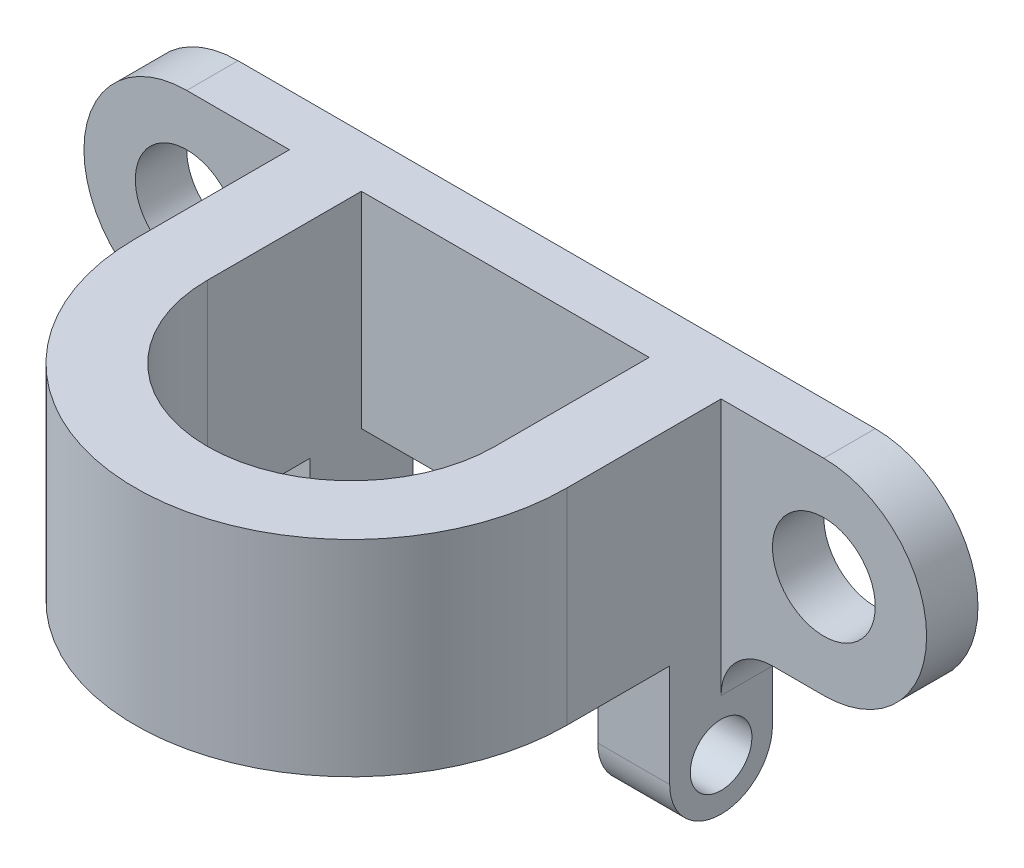
ISO-10303-21;
HEADER;
FILE_DESCRIPTION(('STEP AP214'),'2;1');
FILE_NAME('part.step','',(''),(''),'','','');
FILE_SCHEMA(('AUTOMOTIVE_DESIGN { 1 0 10303 214 1 1 1 1 }'));
ENDSEC;
DATA;
#1=APPLICATION_CONTEXT('core data for automotive mechanical design processes');
#2=APPLICATION_PROTOCOL_DEFINITION('international standard','automotive_design',2000,#1);
#3=PRODUCT_CONTEXT('',#1,'mechanical');
#4=PRODUCT('Part','Part','',(#3));
#5=PRODUCT_RELATED_PRODUCT_CATEGORY('part','',(#4));
#6=PRODUCT_DEFINITION_FORMATION('','',#4);
#7=PRODUCT_DEFINITION_CONTEXT('part definition',#1,'design');
#8=PRODUCT_DEFINITION('design','',#6,#7);
#9=PRODUCT_DEFINITION_SHAPE('','',#8);
#10=(LENGTH_UNIT() NAMED_UNIT(*) SI_UNIT(.MILLI.,.METRE.));
#11=(NAMED_UNIT(*) PLANE_ANGLE_UNIT() SI_UNIT($,.RADIAN.));
#12=(NAMED_UNIT(*) SI_UNIT($,.STERADIAN.) SOLID_ANGLE_UNIT());
#13=UNCERTAINTY_MEASURE_WITH_UNIT(LENGTH_MEASURE(1.E-05),#10,'distance_accuracy_value','');
#14=(GEOMETRIC_REPRESENTATION_CONTEXT(3) GLOBAL_UNCERTAINTY_ASSIGNED_CONTEXT((#13)) GLOBAL_UNIT_ASSIGNED_CONTEXT((#10,
#11,#12)) REPRESENTATION_CONTEXT('',''));
#15=CARTESIAN_POINT('',(0.,0.,0.));
#16=DIRECTION('',(0.,0.,1.));
#17=DIRECTION('',(1.,0.,0.));
#18=AXIS2_PLACEMENT_3D('',#15,#16,#17);
#19=CARTESIAN_POINT('',(0.,-10.,5.));
#20=DIRECTION('',(0.,-1.,0.));
#21=DIRECTION('',(1.,0.,0.));
#22=AXIS2_PLACEMENT_3D('',#19,#20,#21);
#23=PLANE('',#22);
#24=DIRECTION('',(-1.,0.,0.));
#25=VECTOR('',#24,1.);
#26=CARTESIAN_POINT('',(0.,-10.,5.));
#27=LINE('',#26,#25);
#28=CARTESIAN_POINT('',(62.,-10.,5.));
#29=VERTEX_POINT('',#28);
#30=CARTESIAN_POINT('',(57.,-10.,5.));
#31=VERTEX_POINT('',#30);
#32=EDGE_CURVE('E350',#29,#31,#27,.T.);
#33=ORIENTED_EDGE('',*,*,#32,.T.);
#34=DIRECTION('',(0.,0.,1.));
#35=VECTOR('',#34,1.);
#36=CARTESIAN_POINT('',(57.,-10.,0.));
#37=LINE('',#36,#35);
#38=CARTESIAN_POINT('',(57.,-10.,0.));
#39=VERTEX_POINT('',#38);
#40=EDGE_CURVE('E239',#39,#31,#37,.T.);
#41=ORIENTED_EDGE('',*,*,#40,.F.);
#42=DIRECTION('',(-1.,0.,0.));
#43=VECTOR('',#42,1.);
#44=CARTESIAN_POINT('',(0.,-10.,0.));
#45=LINE('',#44,#43);
#46=CARTESIAN_POINT('',(62.,-10.,0.));
#47=VERTEX_POINT('',#46);
#48=EDGE_CURVE('E365',#47,#39,#45,.T.);
#49=ORIENTED_EDGE('',*,*,#48,.F.);
#50=DIRECTION('',(0.,0.,-1.));
#51=VECTOR('',#50,1.);
#52=CARTESIAN_POINT('',(62.,-10.,5.));
#53=LINE('',#52,#51);
#54=EDGE_CURVE('E11',#29,#47,#53,.T.);
#55=ORIENTED_EDGE('',*,*,#54,.F.);
#56=EDGE_LOOP('',(#33,#41,#49,#55));
#57=FACE_BOUND('',#56,.T.);
#58=ADVANCED_FACE('F50',(#57),#23,.T.);
#59=DIRECTION('',(0.,0.,1.));
#60=VECTOR('',#59,1.);
#61=CARTESIAN_POINT('',(45.,-10.,0.));
#62=LINE('',#61,#60);
#63=CARTESIAN_POINT('',(45.,-10.,0.));
#64=VERTEX_POINT('',#63);
#65=CARTESIAN_POINT('',(45.,-10.,5.));
#66=VERTEX_POINT('',#65);
#67=EDGE_CURVE('E250',#64,#66,#62,.T.);
#68=ORIENTED_EDGE('',*,*,#67,.T.);
#69=DIRECTION('',(1.,0.,0.));
#70=VECTOR('',#69,1.);
#71=CARTESIAN_POINT('',(17.,-10.,5.));
#72=LINE('',#71,#70);
#73=CARTESIAN_POINT('',(17.,-10.,5.));
#74=VERTEX_POINT('',#73);
#75=EDGE_CURVE('E303',#74,#66,#72,.T.);
#76=ORIENTED_EDGE('',*,*,#75,.F.);
#77=DIRECTION('',(0.,0.,1.));
#78=VECTOR('',#77,1.);
#79=CARTESIAN_POINT('',(17.,-10.,0.));
#80=LINE('',#79,#78);
#81=CARTESIAN_POINT('',(17.,-10.,0.));
#82=VERTEX_POINT('',#81);
#83=EDGE_CURVE('E273',#82,#74,#80,.T.);
#84=ORIENTED_EDGE('',*,*,#83,.F.);
#85=EDGE_CURVE('E366',#64,#82,#45,.T.);
#86=ORIENTED_EDGE('',*,*,#85,.F.);
#87=EDGE_LOOP('',(#68,#76,#84,#86));
#88=FACE_BOUND('',#87,.T.);
#89=ADVANCED_FACE('F401',(#88),#23,.T.);
#90=DIRECTION('',(0.,0.,1.));
#91=VECTOR('',#90,1.);
#92=CARTESIAN_POINT('',(5.,-10.,0.));
#93=LINE('',#92,#91);
#94=CARTESIAN_POINT('',(5.,-10.,0.));
#95=VERTEX_POINT('',#94);
#96=CARTESIAN_POINT('',(5.,-10.,5.));
#97=VERTEX_POINT('',#96);
#98=EDGE_CURVE('E275',#95,#97,#93,.T.);
#99=ORIENTED_EDGE('',*,*,#98,.T.);
#100=CARTESIAN_POINT('',(0.,-10.,5.));
#101=VERTEX_POINT('',#100);
#102=EDGE_CURVE('E352',#97,#101,#27,.T.);
#103=ORIENTED_EDGE('',*,*,#102,.T.);
#104=DIRECTION('',(0.,0.,-1.));
#105=VECTOR('',#104,1.);
#106=CARTESIAN_POINT('',(0.,-10.,5.));
#107=LINE('',#106,#105);
#108=CARTESIAN_POINT('',(0.,-10.,0.));
#109=VERTEX_POINT('',#108);
#110=EDGE_CURVE('E363',#101,#109,#107,.T.);
#111=ORIENTED_EDGE('',*,*,#110,.T.);
#112=EDGE_CURVE('E338',#95,#109,#45,.T.);
#113=ORIENTED_EDGE('',*,*,#112,.F.);
#114=EDGE_LOOP('',(#99,#103,#111,#113));
#115=FACE_BOUND('',#114,.T.);
#116=ADVANCED_FACE('F408',(#115),#23,.T.);
#117=CARTESIAN_POINT('',(0.,0.,5.));
#118=DIRECTION('',(0.,0.,1.));
#119=DIRECTION('',(1.,0.,0.));
#120=AXIS2_PLACEMENT_3D('',#117,#118,#119);
#121=PLANE('',#120);
#122=DIRECTION('',(0.,-1.,0.));
#123=VECTOR('',#122,1.);
#124=CARTESIAN_POINT('',(52.,9.99999999999999,5.));
#125=LINE('',#124,#123);
#126=CARTESIAN_POINT('',(52.,9.99999999999999,5.));
#127=VERTEX_POINT('',#126);
#128=CARTESIAN_POINT('',(52.,-15.,5.));
#129=VERTEX_POINT('',#128);
#130=EDGE_CURVE('E343',#127,#129,#125,.T.);
#131=ORIENTED_EDGE('',*,*,#130,.T.);
#132=CARTESIAN_POINT('',(57.,-15.,5.));
#133=DIRECTION('',(0.,0.,-1.));
#134=DIRECTION('',(1.,0.,0.));
#135=AXIS2_PLACEMENT_3D('',#132,#133,#134);
#136=CIRCLE('',#135,5.);
#137=EDGE_CURVE('E229',#129,#31,#136,.T.);
#138=ORIENTED_EDGE('',*,*,#137,.T.);
#139=ORIENTED_EDGE('',*,*,#32,.F.);
#140=CARTESIAN_POINT('',(62.,0.,5.));
#141=DIRECTION('',(0.,0.,1.));
#142=DIRECTION('',(1.,0.,0.));
#143=AXIS2_PLACEMENT_3D('',#140,#141,#142);
#144=CIRCLE('',#143,10.);
#145=CARTESIAN_POINT('',(62.,10.,5.));
#146=VERTEX_POINT('',#145);
#147=EDGE_CURVE('E349',#29,#146,#144,.T.);
#148=ORIENTED_EDGE('',*,*,#147,.T.);
#149=DIRECTION('',(1.,0.,0.));
#150=VECTOR('',#149,1.);
#151=CARTESIAN_POINT('',(0.,10.,5.));
#152=LINE('',#151,#150);
#153=EDGE_CURVE('E354',#127,#146,#152,.T.);
#154=ORIENTED_EDGE('',*,*,#153,.F.);
#155=EDGE_LOOP('',(#131,#138,#139,#148,#154));
#156=FACE_BOUND('',#155,.T.);
#157=CARTESIAN_POINT('',(62.,0.,5.));
#158=DIRECTION('',(0.,0.,1.));
#159=DIRECTION('',(1.,0.,0.));
#160=AXIS2_PLACEMENT_3D('',#157,#158,#159);
#161=CIRCLE('',#160,5.);
#162=CARTESIAN_POINT('',(67.,0.,5.));
#163=VERTEX_POINT('',#162);
#164=EDGE_CURVE('E283',#163,#163,#161,.T.);
#165=ORIENTED_EDGE('',*,*,#164,.F.);
#166=EDGE_LOOP('',(#165));
#167=FACE_BOUND('',#166,.T.);
#168=ADVANCED_FACE('F413',(#156,#167),#121,.T.);
#169=DIRECTION('',(-1.,0.,0.));
#170=VECTOR('',#169,1.);
#171=CARTESIAN_POINT('',(52.,-10.,10.));
#172=LINE('',#171,#170);
#173=CARTESIAN_POINT('',(52.,-10.,10.));
#174=VERTEX_POINT('',#173);
#175=CARTESIAN_POINT('',(45.,-10.,10.));
#176=VERTEX_POINT('',#175);
#177=EDGE_CURVE('E63',#174,#176,#172,.T.);
#178=ORIENTED_EDGE('',*,*,#177,.F.);
#179=DIRECTION('',(0.,0.,1.));
#180=VECTOR('',#179,1.);
#181=CARTESIAN_POINT('',(52.,-10.,5.));
#182=LINE('',#181,#180);
#183=CARTESIAN_POINT('',(52.,-10.,20.));
#184=VERTEX_POINT('',#183);
#185=EDGE_CURVE('E334',#174,#184,#182,.T.);
#186=ORIENTED_EDGE('',*,*,#185,.T.);
#187=CARTESIAN_POINT('',(31.,-10.,20.));
#188=DIRECTION('',(0.,-1.,0.));
#189=DIRECTION('',(1.,0.,0.));
#190=AXIS2_PLACEMENT_3D('',#187,#188,#189);
#191=CIRCLE('',#190,21.);
#192=CARTESIAN_POINT('',(10.,-10.,20.));
#193=VERTEX_POINT('',#192);
#194=EDGE_CURVE('E326',#184,#193,#191,.T.);
#195=ORIENTED_EDGE('',*,*,#194,.T.);
#196=DIRECTION('',(0.,0.,-1.));
#197=VECTOR('',#196,1.);
#198=CARTESIAN_POINT('',(10.,-10.,5.));
#199=LINE('',#198,#197);
#200=CARTESIAN_POINT('',(10.,-10.,10.));
#201=VERTEX_POINT('',#200);
#202=EDGE_CURVE('E317',#193,#201,#199,.T.);
#203=ORIENTED_EDGE('',*,*,#202,.T.);
#204=DIRECTION('',(1.,0.,0.));
#205=VECTOR('',#204,1.);
#206=CARTESIAN_POINT('',(10.,-10.,10.));
#207=LINE('',#206,#205);
#208=CARTESIAN_POINT('',(17.,-10.,10.));
#209=VERTEX_POINT('',#208);
#210=EDGE_CURVE('E254',#201,#209,#207,.T.);
#211=ORIENTED_EDGE('',*,*,#210,.T.);
#212=DIRECTION('',(0.,0.,-1.));
#213=VECTOR('',#212,1.);
#214=CARTESIAN_POINT('',(17.,-10.,5.));
#215=LINE('',#214,#213);
#216=CARTESIAN_POINT('',(17.,-10.,20.));
#217=VERTEX_POINT('',#216);
#218=EDGE_CURVE('E291',#217,#209,#215,.T.);
#219=ORIENTED_EDGE('',*,*,#218,.F.);
#220=CARTESIAN_POINT('',(31.,-10.,20.));
#221=DIRECTION('',(0.,-1.,0.));
#222=DIRECTION('',(1.,0.,0.));
#223=AXIS2_PLACEMENT_3D('',#220,#221,#222);
#224=CIRCLE('',#223,14.);
#225=CARTESIAN_POINT('',(45.,-10.,20.));
#226=VERTEX_POINT('',#225);
#227=EDGE_CURVE('E308',#226,#217,#224,.T.);
#228=ORIENTED_EDGE('',*,*,#227,.F.);
#229=DIRECTION('',(0.,0.,1.));
#230=VECTOR('',#229,1.);
#231=CARTESIAN_POINT('',(45.,-10.,5.));
#232=LINE('',#231,#230);
#233=EDGE_CURVE('E67',#176,#226,#232,.T.);
#234=ORIENTED_EDGE('',*,*,#233,.F.);
#235=EDGE_LOOP('',(#178,#186,#195,#203,#211,#219,#228,#234));
#236=FACE_BOUND('',#235,.T.);
#237=ADVANCED_FACE('F47',(#236),#23,.T.);
#238=CARTESIAN_POINT('',(62.,0.,5.));
#239=DIRECTION('',(0.,0.,-1.));
#240=DIRECTION('',(-1.,0.,0.));
#241=AXIS2_PLACEMENT_3D('',#238,#239,#240);
#242=CYLINDRICAL_SURFACE('',#241,10.);
#243=CARTESIAN_POINT('',(62.,0.,0.));
#244=DIRECTION('',(0.,0.,1.));
#245=DIRECTION('',(1.,0.,0.));
#246=AXIS2_PLACEMENT_3D('',#243,#244,#245);
#247=CIRCLE('',#246,10.);
#248=CARTESIAN_POINT('',(62.,10.,0.));
#249=VERTEX_POINT('',#248);
#250=EDGE_CURVE('E362',#47,#249,#247,.T.);
#251=ORIENTED_EDGE('',*,*,#250,.T.);
#252=DIRECTION('',(0.,0.,-1.));
#253=VECTOR('',#252,1.);
#254=CARTESIAN_POINT('',(62.,10.,5.));
#255=LINE('',#254,#253);
#256=EDGE_CURVE('E57',#146,#249,#255,.T.);
#257=ORIENTED_EDGE('',*,*,#256,.F.);
#258=ORIENTED_EDGE('',*,*,#147,.F.);
#259=ORIENTED_EDGE('',*,*,#54,.T.);
#260=EDGE_LOOP('',(#251,#257,#258,#259));
#261=FACE_BOUND('',#260,.T.);
#262=ADVANCED_FACE('F415',(#261),#242,.T.);
#263=CARTESIAN_POINT('',(0.,10.,5.));
#264=DIRECTION('',(0.,1.,0.));
#265=DIRECTION('',(-1.,0.,0.));
#266=AXIS2_PLACEMENT_3D('',#263,#264,#265);
#267=PLANE('',#266);
#268=DIRECTION('',(1.,0.,0.));
#269=VECTOR('',#268,1.);
#270=CARTESIAN_POINT('',(17.,10.,5.));
#271=LINE('',#270,#269);
#272=CARTESIAN_POINT('',(17.,10.,5.));
#273=VERTEX_POINT('',#272);
#274=CARTESIAN_POINT('',(45.,9.99999999999999,5.));
#275=VERTEX_POINT('',#274);
#276=EDGE_CURVE('E289',#273,#275,#271,.T.);
#277=ORIENTED_EDGE('',*,*,#276,.T.);
#278=DIRECTION('',(0.,0.,1.));
#279=VECTOR('',#278,1.);
#280=CARTESIAN_POINT('',(45.,9.99999999999999,5.));
#281=LINE('',#280,#279);
#282=CARTESIAN_POINT('',(45.,10.,20.));
#283=VERTEX_POINT('',#282);
#284=EDGE_CURVE('E292',#275,#283,#281,.T.);
#285=ORIENTED_EDGE('',*,*,#284,.T.);
#286=CARTESIAN_POINT('',(31.,10.,20.));
#287=DIRECTION('',(0.,-1.,0.));
#288=DIRECTION('',(1.,0.,0.));
#289=AXIS2_PLACEMENT_3D('',#286,#287,#288);
#290=CIRCLE('',#289,14.);
#291=CARTESIAN_POINT('',(17.,10.,20.));
#292=VERTEX_POINT('',#291);
#293=EDGE_CURVE('E298',#283,#292,#290,.T.);
#294=ORIENTED_EDGE('',*,*,#293,.T.);
#295=DIRECTION('',(0.,0.,-1.));
#296=VECTOR('',#295,1.);
#297=CARTESIAN_POINT('',(17.,10.,5.));
#298=LINE('',#297,#296);
#299=EDGE_CURVE('E299',#292,#273,#298,.T.);
#300=ORIENTED_EDGE('',*,*,#299,.T.);
#301=EDGE_LOOP('',(#277,#285,#294,#300));
#302=FACE_BOUND('',#301,.T.);
#303=DIRECTION('',(1.,0.,0.));
#304=VECTOR('',#303,1.);
#305=CARTESIAN_POINT('',(0.,10.,0.));
#306=LINE('',#305,#304);
#307=CARTESIAN_POINT('',(0.,10.,0.));
#308=VERTEX_POINT('',#307);
#309=EDGE_CURVE('E367',#308,#249,#306,.T.);
#310=ORIENTED_EDGE('',*,*,#309,.F.);
#311=DIRECTION('',(0.,0.,-1.));
#312=VECTOR('',#311,1.);
#313=CARTESIAN_POINT('',(0.,10.,5.));
#314=LINE('',#313,#312);
#315=CARTESIAN_POINT('',(0.,10.,5.));
#316=VERTEX_POINT('',#315);
#317=EDGE_CURVE('E380',#316,#308,#314,.T.);
#318=ORIENTED_EDGE('',*,*,#317,.F.);
#319=CARTESIAN_POINT('',(10.,10.,5.));
#320=VERTEX_POINT('',#319);
#321=EDGE_CURVE('E351',#316,#320,#152,.T.);
#322=ORIENTED_EDGE('',*,*,#321,.T.);
#323=DIRECTION('',(0.,0.,-1.));
#324=VECTOR('',#323,1.);
#325=CARTESIAN_POINT('',(10.,10.,5.));
#326=LINE('',#325,#324);
#327=CARTESIAN_POINT('',(10.,10.,20.));
#328=VERTEX_POINT('',#327);
#329=EDGE_CURVE('E322',#328,#320,#326,.T.);
#330=ORIENTED_EDGE('',*,*,#329,.F.);
#331=CARTESIAN_POINT('',(31.,10.,20.));
#332=DIRECTION('',(0.,-1.,0.));
#333=DIRECTION('',(1.,0.,0.));
#334=AXIS2_PLACEMENT_3D('',#331,#332,#333);
#335=CIRCLE('',#334,21.);
#336=CARTESIAN_POINT('',(52.,9.99999999999999,20.));
#337=VERTEX_POINT('',#336);
#338=EDGE_CURVE('E327',#337,#328,#335,.T.);
#339=ORIENTED_EDGE('',*,*,#338,.F.);
#340=DIRECTION('',(0.,0.,1.));
#341=VECTOR('',#340,1.);
#342=CARTESIAN_POINT('',(52.,9.99999999999999,5.));
#343=LINE('',#342,#341);
#344=EDGE_CURVE('E324',#127,#337,#343,.T.);
#345=ORIENTED_EDGE('',*,*,#344,.F.);
#346=ORIENTED_EDGE('',*,*,#153,.T.);
#347=ORIENTED_EDGE('',*,*,#256,.T.);
#348=EDGE_LOOP('',(#310,#318,#322,#330,#339,#345,#346,#347));
#349=FACE_BOUND('',#348,.T.);
#350=ADVANCED_FACE('F420',(#302,#349),#267,.T.);
#351=CARTESIAN_POINT('',(0.,0.,5.));
#352=DIRECTION('',(0.,0.,-1.));
#353=DIRECTION('',(-1.,0.,0.));
#354=AXIS2_PLACEMENT_3D('',#351,#352,#353);
#355=CYLINDRICAL_SURFACE('',#354,10.);
#356=CARTESIAN_POINT('',(0.,0.,0.));
#357=DIRECTION('',(0.,0.,1.));
#358=DIRECTION('',(1.,0.,0.));
#359=AXIS2_PLACEMENT_3D('',#356,#357,#358);
#360=CIRCLE('',#359,10.);
#361=EDGE_CURVE('E375',#308,#109,#360,.T.);
#362=ORIENTED_EDGE('',*,*,#361,.T.);
#363=ORIENTED_EDGE('',*,*,#110,.F.);
#364=CARTESIAN_POINT('',(0.,0.,5.));
#365=DIRECTION('',(0.,0.,1.));
#366=DIRECTION('',(1.,0.,0.));
#367=AXIS2_PLACEMENT_3D('',#364,#365,#366);
#368=CIRCLE('',#367,10.);
#369=EDGE_CURVE('E356',#316,#101,#368,.T.);
#370=ORIENTED_EDGE('',*,*,#369,.F.);
#371=ORIENTED_EDGE('',*,*,#317,.T.);
#372=EDGE_LOOP('',(#362,#363,#370,#371));
#373=FACE_BOUND('',#372,.T.);
#374=ADVANCED_FACE('F436',(#373),#355,.T.);
#375=CARTESIAN_POINT('',(5.,-15.,5.));
#376=DIRECTION('',(0.,0.,-1.));
#377=DIRECTION('',(1.,0.,0.));
#378=AXIS2_PLACEMENT_3D('',#375,#376,#377);
#379=CIRCLE('',#378,5.);
#380=CARTESIAN_POINT('',(10.,-15.,5.));
#381=VERTEX_POINT('',#380);
#382=EDGE_CURVE('E258',#97,#381,#379,.T.);
#383=ORIENTED_EDGE('',*,*,#382,.T.);
#384=DIRECTION('',(0.,-1.,0.));
#385=VECTOR('',#384,1.);
#386=CARTESIAN_POINT('',(10.,10.,5.));
#387=LINE('',#386,#385);
#388=EDGE_CURVE('E335',#320,#381,#387,.T.);
#389=ORIENTED_EDGE('',*,*,#388,.F.);
#390=ORIENTED_EDGE('',*,*,#321,.F.);
#391=ORIENTED_EDGE('',*,*,#369,.T.);
#392=ORIENTED_EDGE('',*,*,#102,.F.);
#393=EDGE_LOOP('',(#383,#389,#390,#391,#392));
#394=FACE_BOUND('',#393,.T.);
#395=CARTESIAN_POINT('',(0.,0.,5.));
#396=DIRECTION('',(0.,0.,1.));
#397=DIRECTION('',(1.,0.,0.));
#398=AXIS2_PLACEMENT_3D('',#395,#396,#397);
#399=CIRCLE('',#398,5.);
#400=CARTESIAN_POINT('',(5.,0.,5.));
#401=VERTEX_POINT('',#400);
#402=EDGE_CURVE('E280',#401,#401,#399,.T.);
#403=ORIENTED_EDGE('',*,*,#402,.F.);
#404=EDGE_LOOP('',(#403));
#405=FACE_BOUND('',#404,.T.);
#406=ADVANCED_FACE('F422',(#394,#405),#121,.T.);
#407=CARTESIAN_POINT('',(0.,0.,0.));
#408=DIRECTION('',(0.,0.,1.));
#409=DIRECTION('',(1.,0.,0.));
#410=AXIS2_PLACEMENT_3D('',#407,#408,#409);
#411=PLANE('',#410);
#412=CARTESIAN_POINT('',(62.,0.,0.));
#413=DIRECTION('',(0.,0.,1.));
#414=DIRECTION('',(1.,0.,0.));
#415=AXIS2_PLACEMENT_3D('',#412,#413,#414);
#416=CIRCLE('',#415,5.);
#417=CARTESIAN_POINT('',(67.,0.,0.));
#418=VERTEX_POINT('',#417);
#419=EDGE_CURVE('E306',#418,#418,#416,.T.);
#420=ORIENTED_EDGE('',*,*,#419,.T.);
#421=EDGE_LOOP('',(#420));
#422=FACE_BOUND('',#421,.T.);
#423=CARTESIAN_POINT('',(0.,0.,0.));
#424=DIRECTION('',(0.,0.,1.));
#425=DIRECTION('',(1.,0.,0.));
#426=AXIS2_PLACEMENT_3D('',#423,#424,#425);
#427=CIRCLE('',#426,5.);
#428=CARTESIAN_POINT('',(5.,0.,0.));
#429=VERTEX_POINT('',#428);
#430=EDGE_CURVE('E287',#429,#429,#427,.T.);
#431=ORIENTED_EDGE('',*,*,#430,.T.);
#432=EDGE_LOOP('',(#431));
#433=FACE_BOUND('',#432,.T.);
#434=ORIENTED_EDGE('',*,*,#48,.T.);
#435=CARTESIAN_POINT('',(57.,-15.,0.));
#436=DIRECTION('',(0.,0.,-1.));
#437=DIRECTION('',(1.,0.,0.));
#438=AXIS2_PLACEMENT_3D('',#435,#436,#437);
#439=CIRCLE('',#438,5.);
#440=CARTESIAN_POINT('',(52.,-15.,0.));
#441=VERTEX_POINT('',#440);
#442=EDGE_CURVE('E235',#441,#39,#439,.T.);
#443=ORIENTED_EDGE('',*,*,#442,.F.);
#444=DIRECTION('',(0.,1.,0.));
#445=VECTOR('',#444,1.);
#446=CARTESIAN_POINT('',(52.,-15.,0.));
#447=LINE('',#446,#445);
#448=CARTESIAN_POINT('',(52.,-20.,0.));
#449=VERTEX_POINT('',#448);
#450=EDGE_CURVE('E240',#449,#441,#447,.T.);
#451=ORIENTED_EDGE('',*,*,#450,.F.);
#452=DIRECTION('',(1.,0.,0.));
#453=VECTOR('',#452,1.);
#454=CARTESIAN_POINT('',(52.,-20.,0.));
#455=LINE('',#454,#453);
#456=CARTESIAN_POINT('',(45.,-20.,0.));
#457=VERTEX_POINT('',#456);
#458=EDGE_CURVE('E232',#457,#449,#455,.T.);
#459=ORIENTED_EDGE('',*,*,#458,.F.);
#460=DIRECTION('',(0.,-1.,0.));
#461=VECTOR('',#460,1.);
#462=CARTESIAN_POINT('',(45.,-20.,0.));
#463=LINE('',#462,#461);
#464=EDGE_CURVE('E218',#64,#457,#463,.T.);
#465=ORIENTED_EDGE('',*,*,#464,.F.);
#466=ORIENTED_EDGE('',*,*,#85,.T.);
#467=DIRECTION('',(0.,1.,0.));
#468=VECTOR('',#467,1.);
#469=CARTESIAN_POINT('',(17.,-20.,0.));
#470=LINE('',#469,#468);
#471=CARTESIAN_POINT('',(17.,-20.,0.));
#472=VERTEX_POINT('',#471);
#473=EDGE_CURVE('E269',#472,#82,#470,.T.);
#474=ORIENTED_EDGE('',*,*,#473,.F.);
#475=DIRECTION('',(1.,0.,0.));
#476=VECTOR('',#475,1.);
#477=CARTESIAN_POINT('',(10.,-20.,0.));
#478=LINE('',#477,#476);
#479=CARTESIAN_POINT('',(10.,-20.,0.));
#480=VERTEX_POINT('',#479);
#481=EDGE_CURVE('E270',#480,#472,#478,.T.);
#482=ORIENTED_EDGE('',*,*,#481,.F.);
#483=DIRECTION('',(0.,-1.,0.));
#484=VECTOR('',#483,1.);
#485=CARTESIAN_POINT('',(10.,-15.,0.));
#486=LINE('',#485,#484);
#487=CARTESIAN_POINT('',(10.,-15.,0.));
#488=VERTEX_POINT('',#487);
#489=EDGE_CURVE('E262',#488,#480,#486,.T.);
#490=ORIENTED_EDGE('',*,*,#489,.F.);
#491=CARTESIAN_POINT('',(5.,-15.,0.));
#492=DIRECTION('',(0.,0.,-1.));
#493=DIRECTION('',(1.,0.,0.));
#494=AXIS2_PLACEMENT_3D('',#491,#492,#493);
#495=CIRCLE('',#494,5.);
#496=EDGE_CURVE('E261',#95,#488,#495,.T.);
#497=ORIENTED_EDGE('',*,*,#496,.F.);
#498=ORIENTED_EDGE('',*,*,#112,.T.);
#499=ORIENTED_EDGE('',*,*,#361,.F.);
#500=ORIENTED_EDGE('',*,*,#309,.T.);
#501=ORIENTED_EDGE('',*,*,#250,.F.);
#502=EDGE_LOOP('',(#434,#443,#451,#459,#465,#466,#474,#482,#490,#497,#498,#499,#500,#501));
#503=FACE_BOUND('',#502,.T.);
#504=ADVANCED_FACE('F381',(#422,#433,#503),#411,.F.);
#505=CARTESIAN_POINT('',(10.,10.,5.));
#506=DIRECTION('',(-1.,0.,0.));
#507=DIRECTION('',(0.,-1.,0.));
#508=AXIS2_PLACEMENT_3D('',#505,#506,#507);
#509=PLANE('',#508);
#510=CARTESIAN_POINT('',(10.,-20.,5.));
#511=DIRECTION('',(-1.,0.,0.));
#512=DIRECTION('',(0.,-1.,0.));
#513=AXIS2_PLACEMENT_3D('',#510,#511,#512);
#514=CIRCLE('',#513,3.);
#515=CARTESIAN_POINT('',(10.,-23.,5.));
#516=VERTEX_POINT('',#515);
#517=EDGE_CURVE('E223',#516,#516,#514,.T.);
#518=ORIENTED_EDGE('',*,*,#517,.F.);
#519=EDGE_LOOP('',(#518));
#520=FACE_BOUND('',#519,.T.);
#521=ORIENTED_EDGE('',*,*,#202,.F.);
#522=DIRECTION('',(0.,-1.,0.));
#523=VECTOR('',#522,1.);
#524=CARTESIAN_POINT('',(10.,10.,20.));
#525=LINE('',#524,#523);
#526=EDGE_CURVE('E336',#328,#193,#525,.T.);
#527=ORIENTED_EDGE('',*,*,#526,.F.);
#528=ORIENTED_EDGE('',*,*,#329,.T.);
#529=ORIENTED_EDGE('',*,*,#388,.T.);
#530=DIRECTION('',(0.,0.,1.));
#531=VECTOR('',#530,1.);
#532=CARTESIAN_POINT('',(10.,-15.,0.));
#533=LINE('',#532,#531);
#534=EDGE_CURVE('E277',#488,#381,#533,.T.);
#535=ORIENTED_EDGE('',*,*,#534,.F.);
#536=ORIENTED_EDGE('',*,*,#489,.T.);
#537=CARTESIAN_POINT('',(10.,-20.,5.));
#538=DIRECTION('',(-1.,0.,0.));
#539=DIRECTION('',(0.,-1.,0.));
#540=AXIS2_PLACEMENT_3D('',#537,#538,#539);
#541=CIRCLE('',#540,5.);
#542=CARTESIAN_POINT('',(10.,-20.,10.));
#543=VERTEX_POINT('',#542);
#544=EDGE_CURVE('E217',#480,#543,#541,.T.);
#545=ORIENTED_EDGE('',*,*,#544,.T.);
#546=DIRECTION('',(0.,-1.,0.));
#547=VECTOR('',#546,1.);
#548=CARTESIAN_POINT('',(10.,-20.,10.));
#549=LINE('',#548,#547);
#550=EDGE_CURVE('E249',#201,#543,#549,.T.);
#551=ORIENTED_EDGE('',*,*,#550,.F.);
#552=EDGE_LOOP('',(#521,#527,#528,#529,#535,#536,#545,#551));
#553=FACE_BOUND('',#552,.T.);
#554=ADVANCED_FACE('F461',(#520,#553),#509,.T.);
#555=CARTESIAN_POINT('',(31.,10.,20.));
#556=DIRECTION('',(0.,-1.,0.));
#557=DIRECTION('',(1.,0.,0.));
#558=AXIS2_PLACEMENT_3D('',#555,#556,#557);
#559=CYLINDRICAL_SURFACE('',#558,21.);
#560=ORIENTED_EDGE('',*,*,#194,.F.);
#561=DIRECTION('',(0.,-1.,0.));
#562=VECTOR('',#561,1.);
#563=CARTESIAN_POINT('',(52.,9.99999999999999,20.));
#564=LINE('',#563,#562);
#565=EDGE_CURVE('E341',#337,#184,#564,.T.);
#566=ORIENTED_EDGE('',*,*,#565,.F.);
#567=ORIENTED_EDGE('',*,*,#338,.T.);
#568=ORIENTED_EDGE('',*,*,#526,.T.);
#569=EDGE_LOOP('',(#560,#566,#567,#568));
#570=FACE_BOUND('',#569,.T.);
#571=ADVANCED_FACE('F459',(#570),#559,.T.);
#572=CARTESIAN_POINT('',(52.,9.99999999999999,5.));
#573=DIRECTION('',(1.,0.,0.));
#574=DIRECTION('',(0.,1.,0.));
#575=AXIS2_PLACEMENT_3D('',#572,#573,#574);
#576=PLANE('',#575);
#577=CARTESIAN_POINT('',(52.,-20.,5.));
#578=DIRECTION('',(1.,0.,0.));
#579=DIRECTION('',(0.,1.,0.));
#580=AXIS2_PLACEMENT_3D('',#577,#578,#579);
#581=CIRCLE('',#580,3.);
#582=CARTESIAN_POINT('',(52.,-17.,5.));
#583=VERTEX_POINT('',#582);
#584=EDGE_CURVE('E897',#583,#583,#581,.T.);
#585=ORIENTED_EDGE('',*,*,#584,.F.);
#586=EDGE_LOOP('',(#585));
#587=FACE_BOUND('',#586,.T.);
#588=ORIENTED_EDGE('',*,*,#185,.F.);
#589=DIRECTION('',(0.,1.,0.));
#590=VECTOR('',#589,1.);
#591=CARTESIAN_POINT('',(52.,-10.,10.));
#592=LINE('',#591,#590);
#593=CARTESIAN_POINT('',(52.,-20.,10.));
#594=VERTEX_POINT('',#593);
#595=EDGE_CURVE('E205',#594,#174,#592,.T.);
#596=ORIENTED_EDGE('',*,*,#595,.F.);
#597=CARTESIAN_POINT('',(52.,-20.,5.));
#598=DIRECTION('',(1.,0.,0.));
#599=DIRECTION('',(0.,1.,0.));
#600=AXIS2_PLACEMENT_3D('',#597,#598,#599);
#601=CIRCLE('',#600,5.);
#602=EDGE_CURVE('E215',#594,#449,#601,.T.);
#603=ORIENTED_EDGE('',*,*,#602,.T.);
#604=ORIENTED_EDGE('',*,*,#450,.T.);
#605=DIRECTION('',(0.,0.,1.));
#606=VECTOR('',#605,1.);
#607=CARTESIAN_POINT('',(52.,-15.,0.));
#608=LINE('',#607,#606);
#609=EDGE_CURVE('E243',#441,#129,#608,.T.);
#610=ORIENTED_EDGE('',*,*,#609,.T.);
#611=ORIENTED_EDGE('',*,*,#130,.F.);
#612=ORIENTED_EDGE('',*,*,#344,.T.);
#613=ORIENTED_EDGE('',*,*,#565,.T.);
#614=EDGE_LOOP('',(#588,#596,#603,#604,#610,#611,#612,#613));
#615=FACE_BOUND('',#614,.T.);
#616=ADVANCED_FACE('F454',(#587,#615),#576,.T.);
#617=CARTESIAN_POINT('',(17.,10.,5.));
#618=DIRECTION('',(0.,0.,-1.));
#619=DIRECTION('',(-1.,0.,0.));
#620=AXIS2_PLACEMENT_3D('',#617,#618,#619);
#621=PLANE('',#620);
#622=ORIENTED_EDGE('',*,*,#75,.T.);
#623=DIRECTION('',(0.,-1.,0.));
#624=VECTOR('',#623,1.);
#625=CARTESIAN_POINT('',(45.,9.99999999999999,5.));
#626=LINE('',#625,#624);
#627=EDGE_CURVE('E305',#275,#66,#626,.T.);
#628=ORIENTED_EDGE('',*,*,#627,.F.);
#629=ORIENTED_EDGE('',*,*,#276,.F.);
#630=DIRECTION('',(0.,-1.,0.));
#631=VECTOR('',#630,1.);
#632=CARTESIAN_POINT('',(17.,10.,5.));
#633=LINE('',#632,#631);
#634=EDGE_CURVE('E312',#273,#74,#633,.T.);
#635=ORIENTED_EDGE('',*,*,#634,.T.);
#636=EDGE_LOOP('',(#622,#628,#629,#635));
#637=FACE_BOUND('',#636,.T.);
#638=ADVANCED_FACE('F479',(#637),#621,.F.);
#639=CARTESIAN_POINT('',(17.,10.,5.));
#640=DIRECTION('',(-1.,0.,0.));
#641=DIRECTION('',(0.,-1.,0.));
#642=AXIS2_PLACEMENT_3D('',#639,#640,#641);
#643=PLANE('',#642);
#644=CARTESIAN_POINT('',(17.,-20.,5.));
#645=DIRECTION('',(-1.,0.,0.));
#646=DIRECTION('',(0.,-1.,0.));
#647=AXIS2_PLACEMENT_3D('',#644,#645,#646);
#648=CIRCLE('',#647,3.);
#649=CARTESIAN_POINT('',(17.,-23.,5.));
#650=VERTEX_POINT('',#649);
#651=EDGE_CURVE('E892',#650,#650,#648,.T.);
#652=ORIENTED_EDGE('',*,*,#651,.T.);
#653=EDGE_LOOP('',(#652));
#654=FACE_BOUND('',#653,.T.);
#655=ORIENTED_EDGE('',*,*,#218,.T.);
#656=DIRECTION('',(0.,-1.,0.));
#657=VECTOR('',#656,1.);
#658=CARTESIAN_POINT('',(17.,-20.,10.));
#659=LINE('',#658,#657);
#660=CARTESIAN_POINT('',(17.,-20.,10.));
#661=VERTEX_POINT('',#660);
#662=EDGE_CURVE('E246',#209,#661,#659,.T.);
#663=ORIENTED_EDGE('',*,*,#662,.T.);
#664=CARTESIAN_POINT('',(17.,-20.,5.));
#665=DIRECTION('',(-1.,0.,0.));
#666=DIRECTION('',(0.,-1.,0.));
#667=AXIS2_PLACEMENT_3D('',#664,#665,#666);
#668=CIRCLE('',#667,5.);
#669=EDGE_CURVE('E203',#472,#661,#668,.T.);
#670=ORIENTED_EDGE('',*,*,#669,.F.);
#671=ORIENTED_EDGE('',*,*,#473,.T.);
#672=ORIENTED_EDGE('',*,*,#83,.T.);
#673=ORIENTED_EDGE('',*,*,#634,.F.);
#674=ORIENTED_EDGE('',*,*,#299,.F.);
#675=DIRECTION('',(0.,-1.,0.));
#676=VECTOR('',#675,1.);
#677=CARTESIAN_POINT('',(17.,10.,20.));
#678=LINE('',#677,#676);
#679=EDGE_CURVE('E320',#292,#217,#678,.T.);
#680=ORIENTED_EDGE('',*,*,#679,.T.);
#681=EDGE_LOOP('',(#655,#663,#670,#671,#672,#673,#674,#680));
#682=FACE_BOUND('',#681,.T.);
#683=ADVANCED_FACE('F468',(#654,#682),#643,.F.);
#684=CARTESIAN_POINT('',(31.,10.,20.));
#685=DIRECTION('',(0.,-1.,0.));
#686=DIRECTION('',(1.,0.,0.));
#687=AXIS2_PLACEMENT_3D('',#684,#685,#686);
#688=CYLINDRICAL_SURFACE('',#687,14.);
#689=ORIENTED_EDGE('',*,*,#227,.T.);
#690=ORIENTED_EDGE('',*,*,#679,.F.);
#691=ORIENTED_EDGE('',*,*,#293,.F.);
#692=DIRECTION('',(0.,-1.,0.));
#693=VECTOR('',#692,1.);
#694=CARTESIAN_POINT('',(45.,9.99999999999999,20.));
#695=LINE('',#694,#693);
#696=EDGE_CURVE('E316',#283,#226,#695,.T.);
#697=ORIENTED_EDGE('',*,*,#696,.T.);
#698=EDGE_LOOP('',(#689,#690,#691,#697));
#699=FACE_BOUND('',#698,.T.);
#700=ADVANCED_FACE('F473',(#699),#688,.F.);
#701=CARTESIAN_POINT('',(45.,9.99999999999999,5.));
#702=DIRECTION('',(1.,0.,0.));
#703=DIRECTION('',(0.,1.,0.));
#704=AXIS2_PLACEMENT_3D('',#701,#702,#703);
#705=PLANE('',#704);
#706=CARTESIAN_POINT('',(45.,-20.,5.));
#707=DIRECTION('',(1.,0.,0.));
#708=DIRECTION('',(0.,1.,0.));
#709=AXIS2_PLACEMENT_3D('',#706,#707,#708);
#710=CIRCLE('',#709,3.);
#711=CARTESIAN_POINT('',(45.,-17.,5.));
#712=VERTEX_POINT('',#711);
#713=EDGE_CURVE('E51',#712,#712,#710,.T.);
#714=ORIENTED_EDGE('',*,*,#713,.T.);
#715=EDGE_LOOP('',(#714));
#716=FACE_BOUND('',#715,.T.);
#717=ORIENTED_EDGE('',*,*,#627,.T.);
#718=ORIENTED_EDGE('',*,*,#67,.F.);
#719=ORIENTED_EDGE('',*,*,#464,.T.);
#720=CARTESIAN_POINT('',(45.,-20.,5.));
#721=DIRECTION('',(1.,0.,0.));
#722=DIRECTION('',(0.,1.,0.));
#723=AXIS2_PLACEMENT_3D('',#720,#721,#722);
#724=CIRCLE('',#723,5.);
#725=CARTESIAN_POINT('',(45.,-20.,10.));
#726=VERTEX_POINT('',#725);
#727=EDGE_CURVE('E208',#726,#457,#724,.T.);
#728=ORIENTED_EDGE('',*,*,#727,.F.);
#729=DIRECTION('',(0.,1.,0.));
#730=VECTOR('',#729,1.);
#731=CARTESIAN_POINT('',(45.,-10.,10.));
#732=LINE('',#731,#730);
#733=EDGE_CURVE('E193',#726,#176,#732,.T.);
#734=ORIENTED_EDGE('',*,*,#733,.T.);
#735=ORIENTED_EDGE('',*,*,#233,.T.);
#736=ORIENTED_EDGE('',*,*,#696,.F.);
#737=ORIENTED_EDGE('',*,*,#284,.F.);
#738=EDGE_LOOP('',(#717,#718,#719,#728,#734,#735,#736,#737));
#739=FACE_BOUND('',#738,.T.);
#740=ADVANCED_FACE('F216',(#716,#739),#705,.F.);
#741=CARTESIAN_POINT('',(0.,0.,-15.));
#742=DIRECTION('',(0.,0.,1.));
#743=DIRECTION('',(1.,0.,0.));
#744=AXIS2_PLACEMENT_3D('',#741,#742,#743);
#745=CYLINDRICAL_SURFACE('',#744,5.);
#746=ORIENTED_EDGE('',*,*,#402,.T.);
#747=EDGE_LOOP('',(#746));
#748=FACE_BOUND('',#747,.T.);
#749=ORIENTED_EDGE('',*,*,#430,.F.);
#750=EDGE_LOOP('',(#749));
#751=FACE_BOUND('',#750,.T.);
#752=ADVANCED_FACE('F389',(#748,#751),#745,.F.);
#753=CARTESIAN_POINT('',(62.,0.,-15.));
#754=DIRECTION('',(0.,0.,1.));
#755=DIRECTION('',(1.,0.,0.));
#756=AXIS2_PLACEMENT_3D('',#753,#754,#755);
#757=CYLINDRICAL_SURFACE('',#756,5.);
#758=ORIENTED_EDGE('',*,*,#164,.T.);
#759=EDGE_LOOP('',(#758));
#760=FACE_BOUND('',#759,.T.);
#761=ORIENTED_EDGE('',*,*,#419,.F.);
#762=EDGE_LOOP('',(#761));
#763=FACE_BOUND('',#762,.T.);
#764=ADVANCED_FACE('F390',(#760,#763),#757,.F.);
#765=CARTESIAN_POINT('',(5.,-15.,0.));
#766=DIRECTION('',(0.,0.,1.));
#767=DIRECTION('',(1.,0.,0.));
#768=AXIS2_PLACEMENT_3D('',#765,#766,#767);
#769=CYLINDRICAL_SURFACE('',#768,5.);
#770=ORIENTED_EDGE('',*,*,#382,.F.);
#771=ORIENTED_EDGE('',*,*,#98,.F.);
#772=ORIENTED_EDGE('',*,*,#496,.T.);
#773=ORIENTED_EDGE('',*,*,#534,.T.);
#774=EDGE_LOOP('',(#770,#771,#772,#773));
#775=FACE_BOUND('',#774,.T.);
#776=ADVANCED_FACE('F388',(#775),#769,.F.);
#777=CARTESIAN_POINT('',(10.,-20.,10.));
#778=DIRECTION('',(0.,0.,1.));
#779=DIRECTION('',(1.,0.,0.));
#780=AXIS2_PLACEMENT_3D('',#777,#778,#779);
#781=PLANE('',#780);
#782=ORIENTED_EDGE('',*,*,#662,.F.);
#783=ORIENTED_EDGE('',*,*,#210,.F.);
#784=ORIENTED_EDGE('',*,*,#550,.T.);
#785=DIRECTION('',(1.,0.,0.));
#786=VECTOR('',#785,1.);
#787=CARTESIAN_POINT('',(10.,-20.,10.));
#788=LINE('',#787,#786);
#789=EDGE_CURVE('E256',#543,#661,#788,.T.);
#790=ORIENTED_EDGE('',*,*,#789,.T.);
#791=EDGE_LOOP('',(#782,#783,#784,#790));
#792=FACE_BOUND('',#791,.T.);
#793=ADVANCED_FACE('F400',(#792),#781,.T.);
#794=CARTESIAN_POINT('',(57.,-15.,0.));
#795=DIRECTION('',(0.,0.,1.));
#796=DIRECTION('',(1.,0.,0.));
#797=AXIS2_PLACEMENT_3D('',#794,#795,#796);
#798=CYLINDRICAL_SURFACE('',#797,5.);
#799=ORIENTED_EDGE('',*,*,#137,.F.);
#800=ORIENTED_EDGE('',*,*,#609,.F.);
#801=ORIENTED_EDGE('',*,*,#442,.T.);
#802=ORIENTED_EDGE('',*,*,#40,.T.);
#803=EDGE_LOOP('',(#799,#800,#801,#802));
#804=FACE_BOUND('',#803,.T.);
#805=ADVANCED_FACE('F455',(#804),#798,.F.);
#806=CARTESIAN_POINT('',(52.,-10.,10.));
#807=DIRECTION('',(0.,0.,1.));
#808=DIRECTION('',(1.,0.,0.));
#809=AXIS2_PLACEMENT_3D('',#806,#807,#808);
#810=PLANE('',#809);
#811=ORIENTED_EDGE('',*,*,#733,.F.);
#812=DIRECTION('',(-1.,0.,0.));
#813=VECTOR('',#812,1.);
#814=CARTESIAN_POINT('',(52.,-20.,10.));
#815=LINE('',#814,#813);
#816=EDGE_CURVE('E198',#594,#726,#815,.T.);
#817=ORIENTED_EDGE('',*,*,#816,.F.);
#818=ORIENTED_EDGE('',*,*,#595,.T.);
#819=ORIENTED_EDGE('',*,*,#177,.T.);
#820=EDGE_LOOP('',(#811,#817,#818,#819));
#821=FACE_BOUND('',#820,.T.);
#822=ADVANCED_FACE('F196',(#821),#810,.T.);
#823=CARTESIAN_POINT('',(17.,-20.,5.));
#824=DIRECTION('',(-1.,0.,0.));
#825=DIRECTION('',(0.,-1.,0.));
#826=AXIS2_PLACEMENT_3D('',#823,#824,#825);
#827=CYLINDRICAL_SURFACE('',#826,5.);
#828=ORIENTED_EDGE('',*,*,#544,.F.);
#829=ORIENTED_EDGE('',*,*,#481,.T.);
#830=ORIENTED_EDGE('',*,*,#669,.T.);
#831=ORIENTED_EDGE('',*,*,#789,.F.);
#832=EDGE_LOOP('',(#828,#829,#830,#831));
#833=FACE_BOUND('',#832,.T.);
#834=ADVANCED_FACE('F487',(#833),#827,.T.);
#835=CARTESIAN_POINT('',(45.,-20.,5.));
#836=DIRECTION('',(1.,0.,0.));
#837=DIRECTION('',(0.,1.,0.));
#838=AXIS2_PLACEMENT_3D('',#835,#836,#837);
#839=CYLINDRICAL_SURFACE('',#838,5.);
#840=ORIENTED_EDGE('',*,*,#602,.F.);
#841=ORIENTED_EDGE('',*,*,#816,.T.);
#842=ORIENTED_EDGE('',*,*,#727,.T.);
#843=ORIENTED_EDGE('',*,*,#458,.T.);
#844=EDGE_LOOP('',(#840,#841,#842,#843));
#845=FACE_BOUND('',#844,.T.);
#846=ADVANCED_FACE('F206',(#845),#839,.T.);
#847=CARTESIAN_POINT('',(-18.,-20.,5.));
#848=DIRECTION('',(1.,0.,0.));
#849=DIRECTION('',(0.,1.,0.));
#850=AXIS2_PLACEMENT_3D('',#847,#848,#849);
#851=CYLINDRICAL_SURFACE('',#850,3.);
#852=ORIENTED_EDGE('',*,*,#584,.T.);
#853=EDGE_LOOP('',(#852));
#854=FACE_BOUND('',#853,.T.);
#855=ORIENTED_EDGE('',*,*,#713,.F.);
#856=EDGE_LOOP('',(#855));
#857=FACE_BOUND('',#856,.T.);
#858=ADVANCED_FACE('F492',(#854,#857),#851,.F.);
#859=ORIENTED_EDGE('',*,*,#517,.T.);
#860=EDGE_LOOP('',(#859));
#861=FACE_BOUND('',#860,.T.);
#862=ORIENTED_EDGE('',*,*,#651,.F.);
#863=EDGE_LOOP('',(#862));
#864=FACE_BOUND('',#863,.T.);
#865=ADVANCED_FACE('F536',(#861,#864),#851,.F.);
#866=CLOSED_SHELL('',(#58,#89,#116,#168,#237,#262,#350,#374,#406,#504,#554,#571,#616,#638,#683,
#700,#740,#752,#764,#776,#793,#805,#822,#834,#846,#858,#865));
#867=MANIFOLD_SOLID_BREP('B2',#866);
#868=ADVANCED_BREP_SHAPE_REPRESENTATION('',(#18,#867),#14);
#869=SHAPE_DEFINITION_REPRESENTATION(#9,#868);
ENDSEC;
END-ISO-10303-21;
